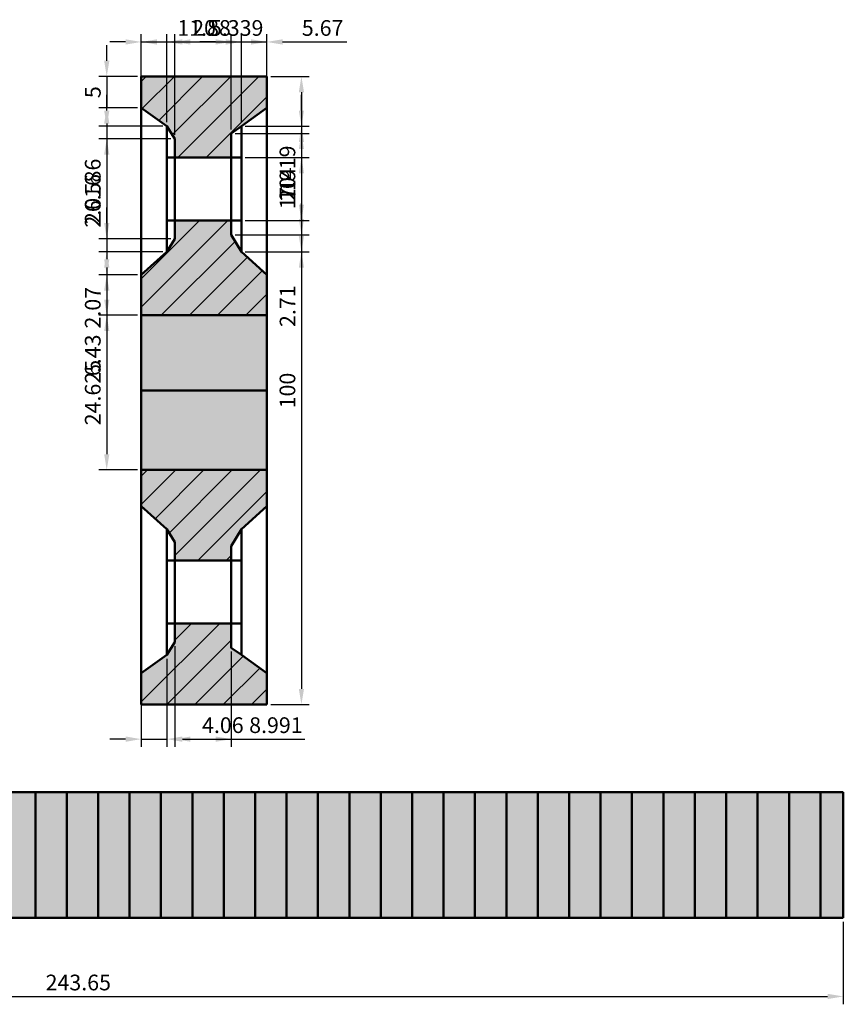
# Model space of a CAD drawing. Units: millimetres. Extents: x 2424 to 2683, y 1522 to 1679.
# Tile 2 of 2: x 2552 to 2683, y 1522 to 1679. Entities that reach past the tile are written whole.
import ezdxf

# ---------------------------------------------------------------- set-up
doc = ezdxf.new("R2010")
doc.units = ezdxf.units.MM
for name, color, linetype, lineweight in [('M-DIMS', 2, 'Continuous', 25), ('M-HATC', 8, 'Continuous', 18), ('M-OUTL', 7, 'Continuous', 50)]:
    doc.layers.add(name, color=color, linetype=linetype, lineweight=lineweight)
doc.styles.get("Standard").update_dxf_attribs({"font": 'arial.ttf'})
doc.dimstyles.new('ISO-25', dxfattribs={"dimtxt": 2.5, "dimasz": 2.5, "dimexe": 1.25, "dimexo": 0.625, "dimtad": 1, "dimtxsty": 'Standard', "dimcen": 2.5, "dimadec": 0, "dimazin": 0, "dimtfac": 1, "dimtmove": 0, "dimatfit": 3, "dimfxl": 1, "dimarcsym": 0})

# ---------------------------------------------------------------- blocks, each defined once
blk = doc.blocks.new('*D11')
at = {"layer": 'Defpoints', "color": 0, "transparency": 16777216}
for p in [(2591.71, 1675.48), (2571.71, 1669.98), (2591.71, 1669.98)]:
    blk.add_point(p, dxfattribs=at)
at = {"layer": 'M-DIMS', "color": 0, "lineweight": -2, "transparency": 16777216}
for p, q in [((2571.71, 1670.61), (2571.71, 1676.73)), ((2591.71, 1670.61), (2591.71, 1676.73)), ((2574.21, 1675.48), (2589.21, 1675.48))]:
    blk.add_line(p, q, dxfattribs=at)
at = {"layer": 'M-DIMS', "color": 0, "transparency": 16777216}
for points in [[(2574.21, 1675.9), (2574.21, 1675.06), (2571.71, 1675.48)], [(2589.21, 1675.9), (2589.21, 1675.06), (2591.71, 1675.48)]]:
    blk.add_solid(points, dxfattribs=at)
at = {"layer": 'M-DIMS', "color": 0, "transparency": 16777216, "insert": (2581.71, 1677.38), "char_height": 2.5, "attachment_point": 5}
blk.add_mtext('20', dxfattribs=at)
blk = doc.blocks.new('*D12')
at = {"layer": 'Defpoints', "color": 0, "transparency": 16777216}
for p in [(2591.71, 1669.98), (2591.71, 1569.98), (2597.21, 1569.98)]:
    blk.add_point(p, dxfattribs=at)
at = {"layer": 'M-DIMS', "color": 0, "lineweight": -2, "transparency": 16777216}
for p, q in [((2592.34, 1669.98), (2598.46, 1669.98)), ((2597.21, 1667.48), (2597.21, 1572.48)), ((2592.34, 1569.98), (2598.46, 1569.98))]:
    blk.add_line(p, q, dxfattribs=at)
at = {"layer": 'M-DIMS', "color": 0, "transparency": 16777216}
for points in [[(2596.8, 1667.48), (2597.63, 1667.48), (2597.21, 1669.98)], [(2596.8, 1572.48), (2597.63, 1572.48), (2597.21, 1569.98)]]:
    blk.add_solid(points, dxfattribs=at)
at = {"layer": 'M-DIMS', "color": 0, "transparency": 16777216, "insert": (2595.31, 1619.98), "char_height": 2.5, "attachment_point": 5, "rotation": 90}
blk.add_mtext('100', dxfattribs=at)
blk = doc.blocks.new('*D13')
at = {"layer": 'Defpoints', "color": 0, "transparency": 16777216}
for p in [(2587.66, 1675.48), (2575.77, 1662.06), (2587.66, 1662.06)]:
    blk.add_point(p, dxfattribs=at)
at = {"layer": 'M-DIMS', "color": 0, "lineweight": -2, "transparency": 16777216}
for p, q in [((2575.77, 1662.69), (2575.77, 1676.73)), ((2587.66, 1662.69), (2587.66, 1676.73)), ((2578.27, 1675.48), (2585.16, 1675.48))]:
    blk.add_line(p, q, dxfattribs=at)
at = {"layer": 'M-DIMS', "color": 0, "transparency": 16777216}
for points in [[(2578.27, 1675.9), (2578.27, 1675.06), (2575.77, 1675.48)], [(2585.16, 1675.9), (2585.16, 1675.06), (2587.66, 1675.48)]]:
    blk.add_solid(points, dxfattribs=at)
at = {"layer": 'M-DIMS', "color": 0, "transparency": 16777216, "insert": (2581.71, 1677.38), "char_height": 2.5, "attachment_point": 5}
blk.add_mtext('11.88', dxfattribs=at)
blk = doc.blocks.new('*D14')
at = {"layer": 'Defpoints', "color": 0, "transparency": 16777216}
for p in [(2577.05, 1579.91), (2586.05, 1579.04), (2586.05, 1564.48)]:
    blk.add_point(p, dxfattribs=at)
at = {"layer": 'M-DIMS', "color": 0, "lineweight": -2, "transparency": 16777216}
for p, q in [((2577.05, 1579.29), (2577.05, 1563.23)), ((2586.05, 1578.41), (2586.05, 1563.23)), ((2579.55, 1564.48), (2583.55, 1564.48)), ((2586.05, 1564.48), (2597.75, 1564.48))]:
    blk.add_line(p, q, dxfattribs=at)
at = {"layer": 'M-DIMS', "color": 0, "transparency": 16777216}
for points in [[(2579.55, 1564.9), (2579.55, 1564.06), (2577.05, 1564.48)], [(2583.55, 1564.9), (2583.55, 1564.06), (2586.05, 1564.48)]]:
    blk.add_solid(points, dxfattribs=at)
at = {"layer": 'M-DIMS', "color": 0, "transparency": 16777216, "insert": (2593.15, 1566.38), "char_height": 2.5, "attachment_point": 5}
blk.add_mtext('8.991', dxfattribs=at)
blk = doc.blocks.new('*D15')
at = {"layer": 'Defpoints', "color": 0, "transparency": 16777216}
for p in [(2575.77, 1577.9), (2571.71, 1574.98), (2575.77, 1564.48)]:
    blk.add_point(p, dxfattribs=at)
at = {"layer": 'M-DIMS', "color": 0, "lineweight": -2, "transparency": 16777216}
for p, q in [((2575.77, 1577.27), (2575.77, 1563.23)), ((2571.71, 1574.36), (2571.71, 1563.23)), ((2569.21, 1564.48), (2566.71, 1564.48)), ((2571.71, 1564.48), (2575.77, 1564.48)), ((2578.27, 1564.48), (2588.62, 1564.48))]:
    blk.add_line(p, q, dxfattribs=at)
at = {"layer": 'M-DIMS', "color": 0, "transparency": 16777216}
for points in [[(2569.21, 1564.9), (2569.21, 1564.06), (2571.71, 1564.48)], [(2578.27, 1564.9), (2578.27, 1564.06), (2575.77, 1564.48)]]:
    blk.add_solid(points, dxfattribs=at)
at = {"layer": 'M-DIMS', "color": 0, "transparency": 16777216, "insert": (2584.7, 1566.38), "char_height": 2.5, "attachment_point": 5}
blk.add_mtext('4.06', dxfattribs=at)
blk = doc.blocks.new('*D16')
at = {"layer": 'Defpoints', "color": 0, "transparency": 16777216}
for p in [(2571.71, 1669.98), (2566.21, 1664.98), (2571.71, 1664.98)]:
    blk.add_point(p, dxfattribs=at)
at = {"layer": 'M-DIMS', "color": 0, "lineweight": -2, "transparency": 16777216}
for p, q in [((2566.21, 1672.48), (2566.21, 1674.98)), ((2571.09, 1669.98), (2564.96, 1669.98)), ((2566.21, 1669.98), (2566.21, 1664.98)), ((2571.09, 1664.98), (2564.96, 1664.98)), ((2566.21, 1662.48), (2566.21, 1659.98))]:
    blk.add_line(p, q, dxfattribs=at)
at = {"layer": 'M-DIMS', "color": 0, "transparency": 16777216}
for points in [[(2565.8, 1672.48), (2566.63, 1672.48), (2566.21, 1669.98)], [(2565.8, 1662.48), (2566.63, 1662.48), (2566.21, 1664.98)]]:
    blk.add_solid(points, dxfattribs=at)
at = {"layer": 'M-DIMS', "color": 0, "transparency": 16777216, "insert": (2564.32, 1667.48), "char_height": 2.5, "attachment_point": 5, "rotation": 90}
blk.add_mtext('5', dxfattribs=at)
blk = doc.blocks.new('*D17')
at = {"layer": 'Defpoints', "color": 0, "transparency": 16777216}
for p in [(2571.71, 1664.98), (2566.21, 1638.39), (2571.71, 1638.39)]:
    blk.add_point(p, dxfattribs=at)
at = {"layer": 'M-DIMS', "color": 0, "lineweight": -2, "transparency": 16777216}
for p, q in [((2571.09, 1664.98), (2564.96, 1664.98)), ((2566.21, 1662.48), (2566.21, 1640.89)), ((2571.09, 1638.39), (2564.96, 1638.39))]:
    blk.add_line(p, q, dxfattribs=at)
at = {"layer": 'M-DIMS', "color": 0, "transparency": 16777216}
for points in [[(2565.8, 1662.48), (2566.63, 1662.48), (2566.21, 1664.98)], [(2565.8, 1640.89), (2566.63, 1640.89), (2566.21, 1638.39)]]:
    blk.add_solid(points, dxfattribs=at)
at = {"layer": 'M-DIMS', "color": 0, "transparency": 16777216, "insert": (2564.31, 1651.69), "char_height": 2.5, "attachment_point": 5, "rotation": 90}
blk.add_mtext('26.586', dxfattribs=at)
blk = doc.blocks.new('*D18')
at = {"layer": 'Defpoints', "color": 0, "transparency": 16777216}
for p in [(2571.71, 1638.39), (2566.21, 1631.96), (2571.71, 1631.96)]:
    blk.add_point(p, dxfattribs=at)
at = {"layer": 'M-DIMS', "color": 0, "lineweight": -2, "transparency": 16777216}
for p, q in [((2571.09, 1638.39), (2564.96, 1638.39)), ((2566.21, 1635.89), (2566.21, 1634.46)), ((2571.09, 1631.96), (2564.96, 1631.96)), ((2566.21, 1631.96), (2566.21, 1621.71))]:
    blk.add_line(p, q, dxfattribs=at)
at = {"layer": 'M-DIMS', "color": 0, "transparency": 16777216}
for points in [[(2565.8, 1635.89), (2566.63, 1635.89), (2566.21, 1638.39)], [(2565.8, 1634.46), (2566.63, 1634.46), (2566.21, 1631.96)]]:
    blk.add_solid(points, dxfattribs=at)
at = {"layer": 'M-DIMS', "color": 0, "transparency": 16777216, "insert": (2564.31, 1625.59), "char_height": 2.5, "attachment_point": 5, "rotation": 90}
blk.add_mtext('6.43', dxfattribs=at)
blk = doc.blocks.new('*D19')
at = {"layer": 'Defpoints', "color": 0, "transparency": 16777216}
for p in [(2571.71, 1631.96), (2566.21, 1607.34), (2571.71, 1607.34)]:
    blk.add_point(p, dxfattribs=at)
at = {"layer": 'M-DIMS', "color": 0, "lineweight": -2, "transparency": 16777216}
for p, q in [((2571.09, 1631.96), (2564.96, 1631.96)), ((2566.21, 1629.46), (2566.21, 1609.84)), ((2571.09, 1607.34), (2564.96, 1607.34))]:
    blk.add_line(p, q, dxfattribs=at)
at = {"layer": 'M-DIMS', "color": 0, "transparency": 16777216}
for points in [[(2565.8, 1629.46), (2566.63, 1629.46), (2566.21, 1631.96)], [(2565.8, 1609.84), (2566.63, 1609.84), (2566.21, 1607.34)]]:
    blk.add_solid(points, dxfattribs=at)
at = {"layer": 'M-DIMS', "color": 0, "transparency": 16777216, "insert": (2564.31, 1619.65), "char_height": 2.5, "attachment_point": 5, "rotation": 90}
blk.add_mtext('24.625', dxfattribs=at)
blk = doc.blocks.new('*D20')
at = {"layer": 'Defpoints', "color": 0, "transparency": 16777216}
for p in [(2591.71, 1669.98), (2587.66, 1662.06), (2597.21, 1662.06)]:
    blk.add_point(p, dxfattribs=at)
at = {"layer": 'M-DIMS', "color": 0, "lineweight": -2, "transparency": 16777216}
for p, q in [((2592.34, 1669.98), (2598.46, 1669.98)), ((2597.21, 1667.48), (2597.21, 1664.56)), ((2588.28, 1662.06), (2598.46, 1662.06)), ((2597.21, 1662.06), (2597.21, 1649.89))]:
    blk.add_line(p, q, dxfattribs=at)
at = {"layer": 'M-DIMS', "color": 0, "transparency": 16777216}
for points in [[(2596.8, 1667.48), (2597.63, 1667.48), (2597.21, 1669.98)], [(2596.8, 1664.56), (2597.63, 1664.56), (2597.21, 1662.06)]]:
    blk.add_solid(points, dxfattribs=at)
at = {"layer": 'M-DIMS', "color": 0, "transparency": 16777216, "insert": (2595.31, 1654.73), "char_height": 2.5, "attachment_point": 5, "rotation": 90}
blk.add_mtext('7.919', dxfattribs=at)
blk = doc.blocks.new('*D21')
at = {"layer": 'Defpoints', "color": 0, "transparency": 16777216}
for p in [(2587.66, 1662.06), (2587.66, 1642.06), (2597.21, 1642.06)]:
    blk.add_point(p, dxfattribs=at)
at = {"layer": 'M-DIMS', "color": 0, "lineweight": -2, "transparency": 16777216}
for p, q in [((2588.28, 1662.06), (2598.46, 1662.06)), ((2597.21, 1659.56), (2597.21, 1644.56)), ((2588.28, 1642.06), (2598.46, 1642.06))]:
    blk.add_line(p, q, dxfattribs=at)
at = {"layer": 'M-DIMS', "color": 0, "transparency": 16777216}
for points in [[(2596.8, 1659.56), (2597.63, 1659.56), (2597.21, 1662.06)], [(2596.8, 1644.56), (2597.63, 1644.56), (2597.21, 1642.06)]]:
    blk.add_solid(points, dxfattribs=at)
at = {"layer": 'M-DIMS', "color": 0, "transparency": 16777216, "insert": (2595.31, 1652.06), "char_height": 2.5, "attachment_point": 5, "rotation": 90}
blk.add_mtext('20', dxfattribs=at)
blk = doc.blocks.new('*D22')
at = {"layer": 'Defpoints', "color": 0, "transparency": 16777216}
for p in [(2587.66, 1657.06), (2587.66, 1647.06), (2597.21, 1647.06)]:
    blk.add_point(p, dxfattribs=at)
at = {"layer": 'M-DIMS', "color": 0, "lineweight": -2, "transparency": 16777216}
for p, q in [((2588.28, 1657.06), (2598.46, 1657.06)), ((2597.21, 1654.56), (2597.21, 1649.56)), ((2588.28, 1647.06), (2598.46, 1647.06))]:
    blk.add_line(p, q, dxfattribs=at)
at = {"layer": 'M-DIMS', "color": 0, "transparency": 16777216}
for points in [[(2596.8, 1654.56), (2597.63, 1654.56), (2597.21, 1657.06)], [(2596.8, 1649.56), (2597.63, 1649.56), (2597.21, 1647.06)]]:
    blk.add_solid(points, dxfattribs=at)
at = {"layer": 'M-DIMS', "color": 0, "transparency": 16777216, "insert": (2595.31, 1652.06), "char_height": 2.5, "attachment_point": 5, "rotation": 90}
blk.add_mtext('10', dxfattribs=at)
blk = doc.blocks.new('*D23')
at = {"layer": 'Defpoints', "color": 0, "transparency": 16777216}
for p in [(2439.85, 1536.01), (2683.5, 1536.01), (2683.5, 1523.51)]:
    blk.add_point(p, dxfattribs=at)
at = {"layer": 'M-DIMS', "color": 0, "lineweight": -2, "transparency": 16777216}
for p, q in [((2439.85, 1535.39), (2439.85, 1522.26)), ((2683.5, 1535.39), (2683.5, 1522.26)), ((2442.35, 1523.51), (2681, 1523.51))]:
    blk.add_line(p, q, dxfattribs=at)
at = {"layer": 'M-DIMS', "color": 0, "transparency": 16777216}
for points in [[(2442.35, 1523.93), (2442.35, 1523.1), (2439.85, 1523.51)], [(2681, 1523.93), (2681, 1523.1), (2683.5, 1523.51)]]:
    blk.add_solid(points, dxfattribs=at)
at = {"layer": 'M-DIMS', "color": 0, "transparency": 16777216, "insert": (2561.68, 1525.41), "char_height": 2.5, "attachment_point": 5}
blk.add_mtext('243.65', dxfattribs=at)
blk = doc.blocks.new('*D26')
at = {"layer": 'Defpoints', "color": 0, "transparency": 16777216}
for p in [(2439.85, 1536.01), (2683.5, 1536.01), (2683.5, 1523.51)]:
    blk.add_point(p, dxfattribs=at)
at = {"layer": 'M-DIMS', "color": 0, "lineweight": -2, "transparency": 16777216}
for p, q in [((2439.85, 1535.39), (2439.85, 1522.26)), ((2683.5, 1535.39), (2683.5, 1522.26)), ((2442.35, 1523.51), (2681, 1523.51))]:
    blk.add_line(p, q, dxfattribs=at)
at = {"layer": 'M-DIMS', "color": 0, "transparency": 16777216}
for points in [[(2442.35, 1523.93), (2442.35, 1523.1), (2439.85, 1523.51)], [(2681, 1523.93), (2681, 1523.1), (2683.5, 1523.51)]]:
    blk.add_solid(points, dxfattribs=at)
at = {"layer": 'M-DIMS', "color": 0, "transparency": 16777216, "insert": (2561.68, 1525.41), "char_height": 2.5, "attachment_point": 5}
blk.add_mtext('243.65', dxfattribs=at)
blk = doc.blocks.new('*D29')
at = {"layer": 'Defpoints', "color": 0, "transparency": 16777216}
for p in [(2577.05, 1675.48), (2571.71, 1664.98), (2577.05, 1660.05)]:
    blk.add_point(p, dxfattribs=at)
at = {"layer": 'M-DIMS', "color": 0, "lineweight": -2, "transparency": 16777216}
for p, q in [((2571.71, 1665.61), (2571.71, 1676.73)), ((2577.05, 1660.67), (2577.05, 1676.73)), ((2569.21, 1675.48), (2566.71, 1675.48)), ((2571.71, 1675.48), (2577.05, 1675.48)), ((2579.55, 1675.48), (2591.75, 1675.48))]:
    blk.add_line(p, q, dxfattribs=at)
at = {"layer": 'M-DIMS', "color": 0, "transparency": 16777216}
for points in [[(2569.21, 1675.9), (2569.21, 1675.06), (2571.71, 1675.48)], [(2579.55, 1675.9), (2579.55, 1675.06), (2577.05, 1675.48)]]:
    blk.add_solid(points, dxfattribs=at)
at = {"layer": 'M-DIMS', "color": 0, "transparency": 16777216, "insert": (2586.9, 1677.38), "char_height": 2.5, "attachment_point": 5}
blk.add_mtext('5.339', dxfattribs=at)
blk = doc.blocks.new('*D30')
at = {"layer": 'Defpoints', "color": 0, "transparency": 16777216}
for p in [(2591.71, 1675.48), (2591.71, 1664.98), (2586.05, 1660.92)]:
    blk.add_point(p, dxfattribs=at)
at = {"layer": 'M-DIMS', "color": 0, "lineweight": -2, "transparency": 16777216}
for p, q in [((2586.05, 1661.55), (2586.05, 1676.73)), ((2591.71, 1665.61), (2591.71, 1676.73)), ((2583.55, 1675.48), (2581.05, 1675.48)), ((2586.05, 1675.48), (2591.71, 1675.48)), ((2594.21, 1675.48), (2604.46, 1675.48))]:
    blk.add_line(p, q, dxfattribs=at)
at = {"layer": 'M-DIMS', "color": 0, "transparency": 16777216}
for points in [[(2583.55, 1675.9), (2583.55, 1675.06), (2586.05, 1675.48)], [(2594.21, 1675.9), (2594.21, 1675.06), (2591.71, 1675.48)]]:
    blk.add_solid(points, dxfattribs=at)
at = {"layer": 'M-DIMS', "color": 0, "transparency": 16777216, "insert": (2600.59, 1677.38), "char_height": 2.5, "attachment_point": 5}
blk.add_mtext('5.67', dxfattribs=at)
blk = doc.blocks.new('*D31')
at = {"layer": 'Defpoints', "color": 0, "transparency": 16777216}
for p in [(2575.77, 1662.06), (2566.21, 1660.05), (2577.05, 1660.05)]:
    blk.add_point(p, dxfattribs=at)
at = {"layer": 'M-DIMS', "color": 0, "lineweight": -2, "transparency": 16777216}
for p, q in [((2566.21, 1664.56), (2566.21, 1667.06)), ((2575.15, 1662.06), (2564.96, 1662.06)), ((2566.21, 1662.06), (2566.21, 1660.05)), ((2576.43, 1660.05), (2564.96, 1660.05)), ((2566.21, 1657.55), (2566.21, 1645.32))]:
    blk.add_line(p, q, dxfattribs=at)
at = {"layer": 'M-DIMS', "color": 0, "transparency": 16777216}
for points in [[(2565.8, 1664.56), (2566.63, 1664.56), (2566.21, 1662.06)], [(2565.8, 1657.55), (2566.63, 1657.55), (2566.21, 1660.05)]]:
    blk.add_solid(points, dxfattribs=at)
at = {"layer": 'M-DIMS', "color": 0, "transparency": 16777216, "insert": (2564.31, 1650.18), "char_height": 2.5, "attachment_point": 5, "rotation": 90}
blk.add_mtext('2.016', dxfattribs=at)
blk = doc.blocks.new('*D32')
at = {"layer": 'Defpoints', "color": 0, "transparency": 16777216}
for p in [(2587.66, 1662.06), (2586.05, 1660.92), (2597.21, 1660.92)]:
    blk.add_point(p, dxfattribs=at)
at = {"layer": 'M-DIMS', "color": 0, "lineweight": -2, "transparency": 16777216}
for p, q in [((2597.21, 1664.56), (2597.21, 1667.06)), ((2588.28, 1662.06), (2598.46, 1662.06)), ((2597.21, 1662.06), (2597.21, 1660.92)), ((2586.67, 1660.92), (2598.46, 1660.92)), ((2597.21, 1658.42), (2597.21, 1648.43))]:
    blk.add_line(p, q, dxfattribs=at)
at = {"layer": 'M-DIMS', "color": 0, "transparency": 16777216}
for points in [[(2596.8, 1664.56), (2597.63, 1664.56), (2597.21, 1662.06)], [(2596.8, 1658.42), (2597.63, 1658.42), (2597.21, 1660.92)]]:
    blk.add_solid(points, dxfattribs=at)
at = {"layer": 'M-DIMS', "color": 0, "transparency": 16777216, "insert": (2595.33, 1652.18), "char_height": 2.5, "attachment_point": 5, "rotation": 90}
blk.add_mtext('1.14', dxfattribs=at)
blk = doc.blocks.new('*D33')
at = {"layer": 'Defpoints', "color": 0, "transparency": 16777216}
for p in [(2577.05, 1644.13), (2566.21, 1642.06), (2575.77, 1642.06)]:
    blk.add_point(p, dxfattribs=at)
at = {"layer": 'M-DIMS', "color": 0, "lineweight": -2, "transparency": 16777216}
for p, q in [((2566.21, 1646.63), (2566.21, 1649.13)), ((2576.43, 1644.13), (2564.96, 1644.13)), ((2566.21, 1644.13), (2566.21, 1642.06)), ((2575.15, 1642.06), (2564.96, 1642.06)), ((2566.21, 1639.56), (2566.21, 1629.27))]:
    blk.add_line(p, q, dxfattribs=at)
at = {"layer": 'M-DIMS', "color": 0, "transparency": 16777216}
for points in [[(2565.8, 1646.63), (2566.63, 1646.63), (2566.21, 1644.13)], [(2565.8, 1639.56), (2566.63, 1639.56), (2566.21, 1642.06)]]:
    blk.add_solid(points, dxfattribs=at)
at = {"layer": 'M-DIMS', "color": 0, "transparency": 16777216, "insert": (2564.31, 1633.17), "char_height": 2.5, "attachment_point": 5, "rotation": 90}
blk.add_mtext('2.07', dxfattribs=at)
blk = doc.blocks.new('*D34')
at = {"layer": 'Defpoints', "color": 0, "transparency": 16777216}
for p in [(2586.05, 1644.77), (2587.66, 1642.06), (2597.21, 1642.06)]:
    blk.add_point(p, dxfattribs=at)
at = {"layer": 'M-DIMS', "color": 0, "lineweight": -2, "transparency": 16777216}
for p, q in [((2597.21, 1647.27), (2597.21, 1649.77)), ((2586.67, 1644.77), (2598.46, 1644.77)), ((2597.21, 1644.77), (2597.21, 1642.06)), ((2588.28, 1642.06), (2598.46, 1642.06)), ((2597.21, 1639.56), (2597.21, 1629.76))]:
    blk.add_line(p, q, dxfattribs=at)
at = {"layer": 'M-DIMS', "color": 0, "transparency": 16777216}
for points in [[(2596.8, 1647.27), (2597.63, 1647.27), (2597.21, 1644.77)], [(2596.8, 1639.56), (2597.63, 1639.56), (2597.21, 1642.06)]]:
    blk.add_solid(points, dxfattribs=at)
at = {"layer": 'M-DIMS', "color": 0, "transparency": 16777216, "insert": (2595.33, 1633.41), "char_height": 2.5, "attachment_point": 5, "rotation": 90}
blk.add_mtext('2.71', dxfattribs=at)

msp = doc.modelspace()

# ---------------------------------------------------------------- hatches: boundary and pattern name
at = {"layer": 'M-HATC'}
h = msp.add_hatch(dxfattribs=at)
h.set_pattern_fill('ANSI31', color=256)
h.paths.add_polyline_path([(2581.7148, 1669.9801), (2571.7148, 1669.9801), (2571.7148, 1664.9801), (2575.7745, 1662.0613), (2577.0539, 1660.0454), (2577.0539, 1657.0613), (2581.7148, 1657.0613)])
h.paths.add_polyline_path([(2591.7148, 1669.9801), (2581.7148, 1669.9801), (2581.7148, 1657.0613), (2586.0452, 1657.0613), (2586.0452, 1660.9248), (2587.6551, 1662.0613), (2591.7148, 1664.9801)])
h.paths.add_polyline_path([(2581.7148, 1647.0613), (2577.0539, 1647.0613), (2577.0539, 1644.1286), (2575.7745, 1642.0613), (2571.7148, 1638.3941), (2571.7148, 1631.9639), (2581.7148, 1631.9639)])
h.paths.add_polyline_path([(2591.7148, 1638.3941), (2587.6551, 1642.0613), (2586.0452, 1644.7716), (2586.0452, 1647.0613), (2581.7148, 1647.0613), (2581.7148, 1631.9639), (2591.7148, 1631.9639)])
h.paths.add_polyline_path([(2591.7148, 1601.5661), (2591.7148, 1607.3393), (2571.7148, 1607.3393), (2571.7148, 1601.5661), (2575.7745, 1597.8988), (2577.0539, 1595.8315), (2577.0539, 1592.8988), (2586.0452, 1592.8988), (2586.0452, 1595.1886), (2587.6551, 1597.8988)])
h.paths.add_polyline_path([(2587.6551, 1577.8988), (2586.0452, 1579.0354), (2586.0452, 1582.8988), (2577.0539, 1582.8988), (2577.0539, 1579.9147), (2575.7745, 1577.8988), (2571.7148, 1574.9801), (2571.7148, 1569.9801), (2591.7148, 1569.9801), (2591.7148, 1574.9801)])
h = msp.add_hatch(color=256, dxfattribs=at)
h.set_gradient(color1=(147, 39, 143), color2=(19, 155, 72))
h.paths.add_polyline_path([(2591.7148, 1631.9639), (2571.7148, 1631.9639), (2571.7148, 1619.9801), (2591.7148, 1619.9801)])
h.paths.add_polyline_path([(2591.7148, 1619.9801), (2571.7148, 1619.9801), (2571.7148, 1607.3393), (2591.7148, 1607.3393)])
h.paths.add_polyline_path([(2587.6551, 1642.0613), (2586.0452, 1644.7716), (2586.0452, 1647.0613), (2577.0539, 1647.0613), (2577.0539, 1644.1286), (2575.7745, 1642.0613), (2571.7148, 1638.3941), (2571.7148, 1631.9639), (2591.7148, 1631.9639), (2591.7148, 1638.3941)])
h.paths.add_polyline_path([(2591.7148, 1669.9801), (2571.7148, 1669.9801), (2571.7148, 1664.9801), (2575.7745, 1662.0613), (2577.0539, 1660.0454), (2577.0539, 1657.0613), (2586.0452, 1657.0613), (2586.0452, 1660.9248), (2587.6551, 1662.0613), (2591.7148, 1664.9801)])
h.paths.add_polyline_path([(2591.7148, 1607.3393), (2571.7148, 1607.3393), (2571.7148, 1601.5661), (2575.7745, 1597.8988), (2577.0539, 1595.8315), (2577.0539, 1592.8988), (2586.0452, 1592.8988), (2586.0452, 1595.1886), (2587.6551, 1597.8988), (2591.7148, 1601.5661)])
h.paths.add_polyline_path([(2587.6551, 1577.8988), (2586.0452, 1579.0354), (2586.0452, 1582.8988), (2577.0539, 1582.8988), (2577.0539, 1579.9147), (2575.7745, 1577.8988), (2571.7148, 1574.9801), (2571.7148, 1569.9801), (2591.7148, 1569.9801), (2591.7148, 1574.9801)])
h = msp.add_hatch(color=256, dxfattribs=at)
h.set_gradient(color1=(255, 0, 0))
h.paths.add_polyline_path([(2444.8516, 1556.0123), (2439.8516, 1556.0123), (2439.8516, 1536.0123), (2444.8516, 1536.0123)])
h.paths.add_polyline_path([(2449.8516, 1556.0123), (2444.8516, 1556.0123), (2444.8516, 1536.0123), (2449.8516, 1536.0123)])
h.paths.add_polyline_path([(2454.8516, 1556.0123), (2449.8516, 1556.0123), (2449.8516, 1536.0123), (2454.8516, 1536.0123)])
h.paths.add_polyline_path([(2459.8516, 1556.0123), (2454.8516, 1556.0123), (2454.8516, 1536.0123), (2459.8516, 1536.0123)])
h.paths.add_polyline_path([(2464.8516, 1556.0123), (2459.8516, 1556.0123), (2459.8516, 1536.0123), (2464.8516, 1536.0123)])
h.paths.add_polyline_path([(2469.8516, 1556.0123), (2464.8516, 1556.0123), (2464.8516, 1536.0123), (2469.8516, 1536.0123)])
h.paths.add_polyline_path([(2474.8516, 1556.0123), (2469.8516, 1556.0123), (2469.8516, 1536.0123), (2474.8516, 1536.0123)])
h.paths.add_polyline_path([(2479.8516, 1556.0123), (2474.8516, 1556.0123), (2474.8516, 1536.0123), (2479.8516, 1536.0123)])
h.paths.add_polyline_path([(2484.8516, 1556.0123), (2479.8516, 1556.0123), (2479.8516, 1536.0123), (2484.8516, 1536.0123)])
h.paths.add_polyline_path([(2489.8516, 1556.0123), (2484.8516, 1556.0123), (2484.8516, 1536.0123), (2489.8516, 1536.0123)])
h.paths.add_polyline_path([(2494.8516, 1556.0123), (2489.8516, 1556.0123), (2489.8516, 1536.0123), (2494.8516, 1536.0123)])
h.paths.add_polyline_path([(2499.8516, 1556.0123), (2494.8516, 1556.0123), (2494.8516, 1536.0123), (2499.8516, 1536.0123)])
h.paths.add_polyline_path([(2504.8516, 1556.0123), (2499.8516, 1556.0123), (2499.8516, 1536.0123), (2504.8516, 1536.0123)])
h.paths.add_polyline_path([(2509.8516, 1556.0123), (2504.8516, 1556.0123), (2504.8516, 1536.0123), (2509.8516, 1536.0123)])
h.paths.add_polyline_path([(2514.8516, 1556.0123), (2509.8516, 1556.0123), (2509.8516, 1536.0123), (2514.8516, 1536.0123)])
h.paths.add_polyline_path([(2519.8516, 1556.0123), (2514.8516, 1556.0123), (2514.8516, 1536.0123), (2519.8516, 1536.0123)])
h.paths.add_polyline_path([(2524.8516, 1556.0123), (2519.8516, 1556.0123), (2519.8516, 1536.0123), (2524.8516, 1536.0123)])
h.paths.add_polyline_path([(2529.8516, 1556.0123), (2524.8516, 1556.0123), (2524.8516, 1536.0123), (2529.8516, 1536.0123)])
h.paths.add_polyline_path([(2534.8516, 1556.0123), (2529.8516, 1556.0123), (2529.8516, 1536.0123), (2534.8516, 1536.0123)])
h.paths.add_polyline_path([(2539.8516, 1556.0123), (2534.8516, 1556.0123), (2534.8516, 1536.0123), (2539.8516, 1536.0123)])
h.paths.add_polyline_path([(2544.8516, 1556.0123), (2539.8516, 1556.0123), (2539.8516, 1536.0123), (2544.8516, 1536.0123)])
h.paths.add_polyline_path([(2549.8516, 1556.0123), (2544.8516, 1556.0123), (2544.8516, 1536.0123), (2549.8516, 1536.0123)])
h.paths.add_polyline_path([(2554.8516, 1556.0123), (2549.8516, 1556.0123), (2549.8516, 1536.0123), (2554.8516, 1536.0123)])
h.paths.add_polyline_path([(2559.8516, 1556.0123), (2554.8516, 1556.0123), (2554.8516, 1536.0123), (2559.8516, 1536.0123)])
h.paths.add_polyline_path([(2564.8516, 1556.0123), (2559.8516, 1556.0123), (2559.8516, 1536.0123), (2564.8516, 1536.0123)])
h.paths.add_polyline_path([(2569.8516, 1556.0123), (2564.8516, 1556.0123), (2564.8516, 1536.0123), (2569.8516, 1536.0123)])
h.paths.add_polyline_path([(2574.8516, 1556.0123), (2569.8516, 1556.0123), (2569.8516, 1536.0123), (2574.8516, 1536.0123)])
h.paths.add_polyline_path([(2579.8516, 1556.0123), (2574.8516, 1556.0123), (2574.8516, 1536.0123), (2579.8516, 1536.0123)])
h.paths.add_polyline_path([(2589.8516, 1556.0123), (2584.8516, 1556.0123), (2584.8516, 1536.0123), (2589.8516, 1536.0123)])
h.paths.add_polyline_path([(2584.8516, 1556.0123), (2579.8516, 1556.0123), (2579.8516, 1536.0123), (2584.8516, 1536.0123)])
h.paths.add_polyline_path([(2594.8516, 1556.0123), (2589.8516, 1556.0123), (2589.8516, 1536.0123), (2594.8516, 1536.0123)])
h.paths.add_polyline_path([(2599.8516, 1556.0123), (2594.8516, 1556.0123), (2594.8516, 1536.0123), (2599.8516, 1536.0123)])
h.paths.add_polyline_path([(2604.8516, 1556.0123), (2599.8516, 1556.0123), (2599.8516, 1536.0123), (2604.8516, 1536.0123)])
h.paths.add_polyline_path([(2609.8516, 1556.0123), (2604.8516, 1556.0123), (2604.8516, 1536.0123), (2609.8516, 1536.0123)])
h.paths.add_polyline_path([(2614.8516, 1556.0123), (2609.8516, 1556.0123), (2609.8516, 1536.0123), (2614.8516, 1536.0123)])
h.paths.add_polyline_path([(2619.8516, 1556.0123), (2614.8516, 1556.0123), (2614.8516, 1536.0123), (2619.8516, 1536.0123)])
h.paths.add_polyline_path([(2624.8516, 1556.0123), (2619.8516, 1556.0123), (2619.8516, 1536.0123), (2624.8516, 1536.0123)])
h.paths.add_polyline_path([(2629.8516, 1556.0123), (2624.8516, 1556.0123), (2624.8516, 1536.0123), (2629.8516, 1536.0123)])
h.paths.add_polyline_path([(2634.8516, 1556.0123), (2629.8516, 1556.0123), (2629.8516, 1536.0123), (2634.8516, 1536.0123)])
h.paths.add_polyline_path([(2639.8516, 1556.0123), (2634.8516, 1556.0123), (2634.8516, 1536.0123), (2639.8516, 1536.0123)])
h.paths.add_polyline_path([(2644.8516, 1556.0123), (2639.8516, 1556.0123), (2639.8516, 1536.0123), (2644.8516, 1536.0123)])
h.paths.add_polyline_path([(2649.8516, 1556.0123), (2644.8516, 1556.0123), (2644.8516, 1536.0123), (2649.8516, 1536.0123)])
h.paths.add_polyline_path([(2654.8516, 1556.0123), (2649.8516, 1556.0123), (2649.8516, 1536.0123), (2654.8516, 1536.0123)])
h.paths.add_polyline_path([(2659.8516, 1556.0123), (2654.8516, 1556.0123), (2654.8516, 1536.0123), (2659.8516, 1536.0123)])
h.paths.add_polyline_path([(2664.8516, 1556.0123), (2659.8516, 1556.0123), (2659.8516, 1536.0123), (2664.8516, 1536.0123)])
h.paths.add_polyline_path([(2669.8516, 1556.0123), (2664.8516, 1556.0123), (2664.8516, 1536.0123), (2669.8516, 1536.0123)])
h.paths.add_polyline_path([(2674.8516, 1556.0123), (2669.8516, 1556.0123), (2669.8516, 1536.0123), (2674.8516, 1536.0123)])
h.paths.add_polyline_path([(2679.8516, 1556.0123), (2674.8516, 1556.0123), (2674.8516, 1536.0123), (2679.8516, 1536.0123)])
h.paths.add_polyline_path([(2683.4993, 1556.0123), (2679.8516, 1556.0123), (2679.8516, 1536.0123), (2683.4993, 1536.0123)])

# ---------------------------------------------------------------- linework, layer by layer
at = {"layer": 'M-OUTL'}
for p, q in [((2571.7148, 1669.9801), (2591.7148, 1669.9801)), ((2571.7148, 1569.9801), (2571.7148, 1669.9801)), ((2591.7148, 1669.9801), (2591.7148, 1569.9801)), ((2591.7148, 1669.9801), (2591.7148, 1669.9801)), ((2591.7148, 1669.9801), (2591.7148, 1664.9801)), ((2591.7148, 1664.9801), (2591.7148, 1669.9801)), ((2571.7148, 1664.9801), (2575.7745, 1662.0613)), ((2591.7148, 1664.9801), (2587.6551, 1662.0613)), ((2575.7745, 1662.0613), (2575.7745, 1657.0613)), ((2575.7745, 1662.0613), (2577.0539, 1660.0454)), ((2587.6551, 1662.0613), (2586.0452, 1660.9248)), ((2587.6551, 1662.0613), (2587.6551, 1657.0613)), ((2587.6551, 1662.0613), (2587.6551, 1659.5613)), ((2586.0452, 1660.9248), (2586.0452, 1644.7716)), ((2577.0539, 1660.0454), (2577.0539, 1644.1286)), ((2575.7745, 1657.0613), (2575.7745, 1647.0613)), ((2575.7745, 1657.0613), (2587.6551, 1657.0613)), ((2587.6551, 1657.0613), (2587.6551, 1647.0613)), ((2587.6551, 1657.0613), (2587.6551, 1647.0613)), ((2575.7745, 1647.0613), (2575.7745, 1642.0613)), ((2587.6551, 1647.0613), (2575.7745, 1647.0613)), ((2587.6551, 1647.0613), (2587.6551, 1642.0613)), ((2586.0452, 1644.7716), (2587.6551, 1642.0613)), ((2577.0539, 1644.1286), (2575.7745, 1642.0613)), ((2575.7745, 1642.0613), (2571.7148, 1638.3941)), ((2587.6551, 1642.0613), (2591.7148, 1638.3941)), ((2571.7148, 1631.9639), (2591.7148, 1631.9639)), ((2571.7148, 1619.9801), (2591.7148, 1619.9801)), ((2571.7148, 1607.3393), (2591.7148, 1607.3393)), ((2575.7745, 1597.8988), (2571.7148, 1601.5661)), ((2587.6551, 1597.8988), (2591.7148, 1601.5661)), ((2575.7745, 1592.8988), (2575.7745, 1597.8988)), ((2577.0539, 1595.8315), (2575.7745, 1597.8988)), ((2586.0452, 1595.1886), (2587.6551, 1597.8988)), ((2587.6551, 1592.8988), (2587.6551, 1597.8988)), ((2577.0539, 1579.9147), (2577.0539, 1595.8315)), ((2586.0452, 1579.0354), (2586.0452, 1595.1886)), ((2575.7745, 1582.8988), (2575.7745, 1592.8988)), ((2587.6551, 1592.8988), (2575.7745, 1592.8988)), ((2587.6551, 1582.8988), (2587.6551, 1592.8988)), ((2587.6551, 1582.8988), (2587.6551, 1592.8988)), ((2575.7745, 1577.8988), (2575.7745, 1582.8988)), ((2575.7745, 1582.8988), (2587.6551, 1582.8988)), ((2587.6551, 1577.8988), (2587.6551, 1582.8988)), ((2587.6551, 1577.8988), (2587.6551, 1580.3988)), ((2575.7745, 1577.8988), (2577.0539, 1579.9147)), ((2587.6551, 1577.8988), (2586.0452, 1579.0354)), ((2571.7148, 1574.9801), (2575.7745, 1577.8988)), ((2591.7148, 1574.9801), (2587.6551, 1577.8988)), ((2591.7148, 1569.9801), (2571.7148, 1569.9801)), ((2439.8516, 1556.0123), (2683.4993, 1556.0123)), ((2554.8516, 1556.0123), (2554.8516, 1536.0123)), ((2559.8516, 1536.0123), (2559.8516, 1556.0123)), ((2564.8516, 1556.0123), (2564.8516, 1536.0123)), ((2569.8516, 1536.0123), (2569.8516, 1556.0123)), ((2574.8516, 1556.0123), (2574.8516, 1536.0123)), ((2579.8516, 1536.0123), (2579.8516, 1556.0123)), ((2584.8516, 1556.0123), (2584.8516, 1536.0123)), ((2589.8516, 1536.0123), (2589.8516, 1556.0123)), ((2594.8516, 1556.0123), (2594.8516, 1536.0123)), ((2599.8516, 1536.0123), (2599.8516, 1556.0123)), ((2604.8516, 1556.0123), (2604.8516, 1536.0123)), ((2609.8516, 1536.0123), (2609.8516, 1556.0123)), ((2614.8516, 1556.0123), (2614.8516, 1536.0123)), ((2619.8516, 1536.0123), (2619.8516, 1556.0123)), ((2624.8516, 1556.0123), (2624.8516, 1536.0123)), ((2629.8516, 1536.0123), (2629.8516, 1556.0123)), ((2634.8516, 1556.0123), (2634.8516, 1536.0123)), ((2639.8516, 1536.0123), (2639.8516, 1556.0123)), ((2644.8516, 1556.0123), (2644.8516, 1536.0123)), ((2649.8516, 1536.0123), (2649.8516, 1556.0123)), ((2654.8516, 1556.0123), (2654.8516, 1536.0123)), ((2659.8516, 1536.0123), (2659.8516, 1556.0123)), ((2664.8516, 1556.0123), (2664.8516, 1536.0123)), ((2669.8516, 1536.0123), (2669.8516, 1556.0123)), ((2674.8516, 1556.0123), (2674.8516, 1536.0123)), ((2679.8516, 1536.0123), (2679.8516, 1556.0123)), ((2683.4993, 1556.0123), (2683.4993, 1536.0123)), ((2683.4993, 1536.0123), (2439.8516, 1536.0123))]:
    msp.add_line(p, q, dxfattribs=at)

# ---------------------------------------------------------------- dimensions: what is measured, and where the dimension line sits
at = {"layer": 'M-DIMS'}
for base, p1, p2, override, picture, middle in [((2577.0539, 1675.4801), (2571.7148, 1664.9801), (2577.0539, 1660.0454), {"dimdec": 3, "dimlfac": 1, "dimrnd": 0, "dimzin": 0, "dimdsep": 46, "dimlunit": 2}, '*D29', (2586.8995, 1677.3824)), ((2591.7148, 1675.4801), (2571.7148, 1669.9801), (2591.7148, 1669.9801), {"dimdec": 0, "dimlfac": 1, "dimrnd": 0, "dimzin": 0, "dimdsep": 46, "dimlunit": 2}, '*D11', (2581.7148, 1677.3815)), ((2587.6551, 1675.4801), (2575.7745, 1662.0613), (2587.6551, 1662.0613), {"dimdec": 2, "dimlfac": 1, "dimrnd": 0, "dimzin": 0, "dimdsep": 46, "dimlunit": 2}, '*D13', (2581.7148, 1677.3815)), ((2591.7148, 1675.4801), (2586.0452, 1660.9248), (2591.7148, 1664.9801), {"dimdec": 2, "dimlfac": 1, "dimrnd": 0, "dimzin": 0, "dimdsep": 46, "dimlunit": 2}, '*D30', (2600.5867, 1677.3815)), ((2586.0452, 1564.4801), (2577.0539, 1579.9147), (2586.0452, 1579.0354), {"dimdec": 3, "dimlfac": 1, "dimrnd": 0, "dimzin": 0, "dimdsep": 46, "dimlunit": 2}, '*D14', (2593.1487, 1566.3815)), ((2575.7745, 1564.4801), (2571.7148, 1574.9801), (2575.7745, 1577.8988), {"dimdec": 2, "dimlfac": 1, "dimrnd": 0, "dimzin": 0, "dimdsep": 46, "dimlunit": 2}, '*D15', (2584.6959, 1566.3815)), ((2683.4993, 1523.5123), (2439.8516, 1536.0123), (2683.4993, 1536.0123), {"dimdec": 2, "dimlfac": 1, "dimrnd": 0, "dimzin": 0, "dimdsep": 46, "dimlunit": 2}, '*D23', (2561.6754, 1525.4146)), ((2683.4993, 1523.5123), (2439.8516, 1536.0123), (2683.4993, 1536.0123), {"dimdec": 2, "dimlfac": 1, "dimrnd": 0, "dimzin": 0, "dimdsep": 46, "dimlunit": 2}, '*D26', (2561.6754, 1525.4146))]:
    dim = msp.add_linear_dim(base=base, p1=p1, p2=p2, dimstyle='ISO-25', override=override, dxfattribs=at)
    dim.commit()
    dim.dimension.update_dxf_attribs({"geometry": picture, "text_midpoint": middle})
for base, p1, p2, override, picture, middle in [((2566.2148, 1664.9801), (2571.7148, 1669.9801), (2571.7148, 1664.9801), {"dimdec": 0, "dimlfac": 1, "dimrnd": 0, "dimzin": 0, "dimdsep": 46, "dimlunit": 2}, '*D16', (2564.3185, 1667.4801)), ((2597.2148, 1662.0613), (2591.7148, 1669.9801), (2587.6551, 1662.0613), {"dimdec": 3, "dimlfac": 1, "dimrnd": 0, "dimzin": 0, "dimdsep": 46, "dimlunit": 2}, '*D20', (2595.3134, 1654.7259)), ((2597.2148, 1569.9801), (2591.7148, 1669.9801), (2591.7148, 1569.9801), {"dimdec": 0, "dimlfac": 1, "dimrnd": 0, "dimzin": 0, "dimdsep": 46, "dimlunit": 2}, '*D12', (2595.3134, 1619.9801)), ((2566.2148, 1660.0454), (2575.7745, 1662.0613), (2577.0539, 1660.0454), {"dimdec": 3, "dimlfac": 1, "dimrnd": 0, "dimzin": 0, "dimdsep": 46, "dimlunit": 2}, '*D31', (2564.3134, 1650.1819)), ((2597.2148, 1660.9248), (2587.6551, 1662.0613), (2586.0452, 1660.9248), {"dimdec": 2, "dimlfac": 1, "dimrnd": 0, "dimzin": 0, "dimdsep": 46, "dimlunit": 2}, '*D32', (2595.3347, 1652.1756)), ((2566.2148, 1638.3941), (2571.7148, 1664.9801), (2571.7148, 1638.3941), {"dimdec": 3, "dimlfac": 1, "dimrnd": 0, "dimzin": 0, "dimdsep": 46, "dimlunit": 2}, '*D17', (2564.3134, 1651.6871)), ((2597.2148, 1642.0613), (2587.6551, 1662.0613), (2587.6551, 1642.0613), {"dimdec": 0, "dimlfac": 1, "dimrnd": 0, "dimzin": 0, "dimdsep": 46, "dimlunit": 2}, '*D21', (2595.3134, 1652.0613)), ((2597.2148, 1647.0613), (2587.6551, 1657.0613), (2587.6551, 1647.0613), {"dimdec": 0, "dimlfac": 1, "dimrnd": 0, "dimzin": 0, "dimdsep": 46, "dimlunit": 2}, '*D22', (2595.3134, 1652.0613)), ((2566.2148, 1642.0613), (2577.0539, 1644.1286), (2575.7745, 1642.0613), {"dimdec": 2, "dimlfac": 1, "dimrnd": 0, "dimzin": 0, "dimdsep": 46, "dimlunit": 2}, '*D33', (2564.3134, 1633.1681)), ((2597.2148, 1642.0613), (2586.0452, 1644.7716), (2587.6551, 1642.0613), {"dimdec": 2, "dimlfac": 1, "dimrnd": 0, "dimzin": 0, "dimdsep": 46, "dimlunit": 2}, '*D34', (2595.3347, 1633.4094)), ((2566.2148, 1631.9639), (2571.7148, 1638.3941), (2571.7148, 1631.9639), {"dimdec": 2, "dimlfac": 1, "dimrnd": 0, "dimzin": 0, "dimdsep": 46, "dimlunit": 2}, '*D18', (2564.3125, 1625.5851)), ((2566.2148, 1607.3393), (2571.7148, 1631.9639), (2571.7148, 1607.3393), {"dimdec": 3, "dimlfac": 1, "dimrnd": 0, "dimzin": 0, "dimdsep": 46, "dimlunit": 2}, '*D19', (2564.3134, 1619.6516))]:
    dim = msp.add_linear_dim(base=base, p1=p1, p2=p2, angle=90, dimstyle='ISO-25', override=override, dxfattribs=at)
    dim.commit()
    dim.dimension.update_dxf_attribs({"geometry": picture, "text_midpoint": middle})

doc.saveas('drawing.dxf')
